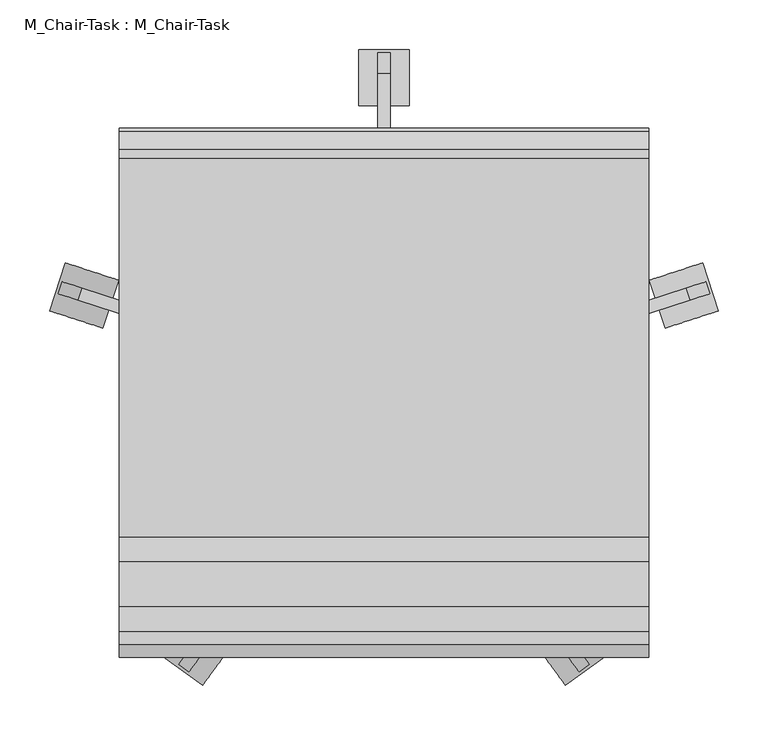
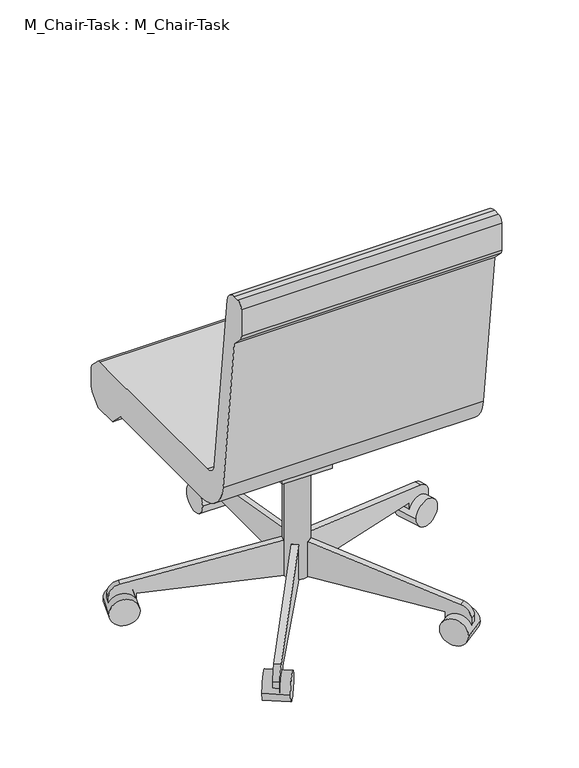
"""IFC4 building model written with IfcOpenShell, lengths in millimetres: furniture geometry, M_Chair-Task : M_Chair-Task."""

from ifc_helpers import new_model, si_unit, point, frame, frame_2d, origin, place, context, project, spatial, polyline, circle_curve, trimmed, segment, composite_curve, outline, extrude, source, transform, mapped, element, save


def m_chair_task_m_chair_task_9903d5c1(model_context):
    return source(origin(), model_context, "Body", "SweptSolid", [
        extrude(outline(composite_curve([segment(polyline([(-126.2050455, 457.2), (255.0102301, 457.2)]), True, "CONTINUOUS"), segment(trimmed(circle_curve(frame_2d((255.0102301, 444.5)), 12.7), [point((255.0102301, 457.2))], [point((263.9604301, 453.510212))], False, "CARTESIAN"), True, "CONTINUOUS"), segment(polyline([(263.9604301, 453.510212), (281.8961016, 435.6939999)]), True, "CONTINUOUS"), segment(trimmed(circle_curve(frame_2d((272.9459016, 426.6837879)), 12.7), [point((281.8961016, 435.6939999))], [point((285.6459016, 426.6837879))], False, "CARTESIAN"), True, "CONTINUOUS"), segment(polyline([(285.6459016, 426.6837879), (285.6459016, 391.6405184)]), True, "CONTINUOUS"), segment(trimmed(circle_curve(frame_2d((260.2459016, 391.6405184)), 25.4), [point((285.6459016, 391.6405184))], [point((278.2663256, 373.7401184))], False, "CARTESIAN"), True, "CONTINUOUS"), segment(polyline([(278.2663256, 373.7401184), (260.2470284, 355.6), (209.4470284, 355.6), (181.0744602, 383.7835944), (-107.1089978, 383.7835944)]), True, "CONTINUOUS"), segment(trimmed(circle_curve(frame_2d((-107.1089978, 459.9835944)), 76.2), [point((-107.1089978, 383.7835944))], [point((-182.7870738, 451.0802913))], False, "CARTESIAN"), True, "CONTINUOUS"), segment(polyline([(-182.7870738, 451.0802913), (-222.3540984, 787.4), (-244.0343545, 809.0802561)]), True, "CONTINUOUS"), segment(trimmed(circle_curve(frame_2d((-235.0540984, 818.0605122)), 12.7), [point((-244.0343545, 809.0802561))], [point((-247.7540984, 818.0605122))], False, "CARTESIAN"), True, "CONTINUOUS"), segment(polyline([(-247.7540984, 818.0605122), (-247.7540984, 876.3)]), True, "CONTINUOUS"), segment(trimmed(circle_curve(frame_2d((-235.0540984, 876.3)), 12.7), [point((-247.7540984, 876.3))], [point((-235.0540984, 889.0))], False, "CARTESIAN"), True, "CONTINUOUS"), segment(polyline([(-235.0540984, 889.0), (-222.1789239, 889.0)]), True, "CONTINUOUS"), segment(trimmed(circle_curve(frame_2d((-222.1789239, 863.6)), 25.4), [point((-222.1789239, 889.0))], [point((-196.9528985, 866.5677677))], False, "CARTESIAN"), True, "CONTINUOUS"), segment(polyline([(-196.9528985, 866.5677677), (-151.4310708, 479.6322323)]), True, "CONTINUOUS"), segment(trimmed(circle_curve(frame_2d((-126.2050455, 482.6)), 25.4), [point((-151.4310708, 479.6322323))], [point((-126.2050455, 457.2))], True, "CARTESIAN"), True, "CONTINUOUS")], self_intersect=False)), frame((-125.7091803, 0.0, 0.0), z_axis=(1.0, 0.0, 0.0), x_axis=(0.0, 1.0, 0.0)), (0.0, 0.0, 1.0), 533.4),
        extrude(outline(polyline([(69.7459016, 383.7835944), (69.7459016, 371.0835944), (18.9459016, 283.0954134), (-19.1540984, 283.0954134), (-19.1540984, 383.7835944), (69.7459016, 383.7835944)])), frame((90.1908197, 0.0, 0.0), z_axis=(1.0, 0.0, 0.0), x_axis=(0.0, 1.0, 0.0)), (0.0, 0.0, 1.0), 101.6),
        extrude(outline(composite_curve([segment(polyline([(311.0459016, 53.5835944), (18.9459016, 53.5835944), (18.9459016, 129.7835944), (44.3459016, 129.7835944), (340.8565654, 77.5007643)]), True, "CONTINUOUS"), segment(trimmed(circle_curve(frame_2d((336.4459016, 52.4866474)), 25.4), [point((340.8565654, 77.5007643))], [point((361.8459016, 52.4866474))], False, "CARTESIAN"), True, "CONTINUOUS"), segment(polyline([(361.8459016, 52.4866474), (361.8459016, 28.1835944), (311.0459016, 28.1835944), (311.0459016, 53.5835944)]), True, "CONTINUOUS")], self_intersect=False)), frame((134.6408197, 0.0, 0.0), z_axis=(1.0, 0.0, 0.0), x_axis=(0.0, 1.0, 0.0)), (0.0, 0.0, 1.0), 12.7),
        extrude(outline(composite_curve([segment(trimmed(circle_curve(frame_2d((336.4459016, 28.1835944)), 28.2002727), [point((308.2456289, 28.1835944))], [point((364.6461744, 28.1835944))], False, "CARTESIAN"), True, "CONTINUOUS"), segment(trimmed(circle_curve(frame_2d((336.4459016, 28.1835944)), 28.2002727), [point((364.6461744, 28.1835944))], [point((308.2456289, 28.1835944))], False, "CARTESIAN"), True, "CONTINUOUS")], self_intersect=False)), frame((115.5908197, 0.0, 0.0), z_axis=(1.0, 0.0, 0.0), x_axis=(0.0, 1.0, 0.0)), (0.0, 0.0, 1.0), 50.8),
        extrude(outline(composite_curve([segment(polyline([(25.4, 0.0), (25.4, 292.1000001), (101.6, 292.1000001), (101.6, 266.7), (49.3171699, -29.8106636)]), True, "CONTINUOUS"), segment(trimmed(circle_curve(frame_2d((24.303053, -25.4)), 25.4), [point((49.3171699, -29.8106636))], [point((24.303053, -50.8))], False, "CARTESIAN"), True, "CONTINUOUS"), segment(polyline([(24.303053, -50.8), (0.0, -50.8), (0.0, 0.0), (25.4, 0.0)]), True, "CONTINUOUS")], self_intersect=False)), frame((-138.7750467, 103.1705568, 28.1835944), z_axis=(0.3090169943749487, 0.9510565162951532, 0.0), x_axis=(0.0, 0.0, 1.0)), (0.0, 0.0, 1.0), 12.7),
        extrude(outline(composite_curve([segment(trimmed(circle_curve(frame_2d((0.0, -28.2002727)), 28.2002727), [point((0.0, -56.4005454))], [point((0.0, 0.0))], False, "CARTESIAN"), True, "CONTINUOUS"), segment(trimmed(circle_curve(frame_2d((0.0, -28.2002727)), 28.2002727), [point((0.0, 0.0))], [point((0.0, -56.4005454))], False, "CARTESIAN"), True, "CONTINUOUS")], self_intersect=False)), frame((-195.638709, 101.6163254, 28.1835944), z_axis=(0.3090169943749487, 0.9510565162951532, 0.0), x_axis=(0.0, 0.0, -1.0)), (0.0, 0.0, 1.0), 50.8),
        extrude(outline(composite_curve([segment(polyline([(25.4, 0.0), (25.4, 292.1), (101.6, 292.1), (101.6, 266.7), (49.3171699, -29.8106637)]), True, "CONTINUOUS"), segment(trimmed(circle_curve(frame_2d((24.303053, -25.3999999)), 25.4), [point((49.3171699, -29.8106637))], [point((24.303053, -50.8))], False, "CARTESIAN"), True, "CONTINUOUS"), segment(polyline([(24.303053, -50.8), (0.0, -50.8), (0.0, 0.0), (25.4, 0.0)]), True, "CONTINUOUS")], self_intersect=False)), frame((-25.5639946, -221.1003988, 28.1835944), z_axis=(-0.8090169943749459, 0.5877852522924754, 0.0), x_axis=(0.0, 0.0, 1.0)), (0.0, 0.0, 1.0), 12.7),
        extrude(outline(composite_curve([segment(trimmed(circle_curve(frame_2d((0.0, -28.2002727)), 28.2002727), [point((0.0, -56.4005455))], [point((0.0, 0.0))], False, "CARTESIAN"), True, "CONTINUOUS"), segment(trimmed(circle_curve(frame_2d((0.0, -28.2002727)), 28.2002727), [point((0.0, 0.0))], [point((0.0, -56.4005455))], False, "CARTESIAN"), True, "CONTINUOUS")], self_intersect=False)), frame((-41.6576707, -275.6612394, 28.1835944), z_axis=(-0.8090169943749458, 0.5877852522924754, 0.0), x_axis=(0.0, 0.0, -1.0)), (0.0, 0.0, 1.0), 50.8),
        extrude(outline(composite_curve([segment(polyline([(-25.4, 0.0), (0.0, 0.0), (0.0, -50.8), (-24.303053, -50.8)]), True, "CONTINUOUS"), segment(trimmed(circle_curve(frame_2d((-24.303053, -25.3999999)), 25.4), [point((-24.303053, -50.8))], [point((-49.3171699, -29.8106636))], False, "CARTESIAN"), True, "CONTINUOUS"), segment(polyline([(-49.3171699, -29.8106636), (-101.6, 266.7), (-101.6, 292.1), (-25.4, 292.1), (-25.4, 0.0)]), True, "CONTINUOUS")], self_intersect=False)), frame((307.545634, -221.1003988, 28.1835944), z_axis=(0.8090169943749499, 0.5877852522924699, 0.0), x_axis=(0.0, 0.0, -1.0)), (0.0, 0.0, 1.0), 12.7),
        extrude(outline(composite_curve([segment(trimmed(circle_curve(frame_2d((0.0, -28.2002727)), 28.2002727), [point((0.0, -56.4005455))], [point((0.0, 0.0))], False, "CARTESIAN"), True, "CONTINUOUS"), segment(trimmed(circle_curve(frame_2d((0.0, -28.2002727)), 28.2002727), [point((0.0, 0.0))], [point((0.0, -56.4005455))], False, "CARTESIAN"), True, "CONTINUOUS")], self_intersect=False)), frame((323.63931, -275.6612394, 28.1835944), z_axis=(0.8090169943749499, 0.5877852522924699, 0.0), x_axis=(0.0, 0.0, 1.0)), (0.0, 0.0, 1.0), 50.8),
        extrude(outline(composite_curve([segment(polyline([(-25.4, 0.0), (0.0, 0.0), (0.0, -50.8), (-24.303053, -50.8)]), True, "CONTINUOUS"), segment(trimmed(circle_curve(frame_2d((-24.303053, -25.4)), 25.4), [point((-24.303053, -50.8))], [point((-49.3171699, -29.8106637))], False, "CARTESIAN"), True, "CONTINUOUS"), segment(polyline([(-49.3171699, -29.8106637), (-101.6, 266.7), (-101.6, 292.1), (-25.4, 292.1), (-25.4, 0.0)]), True, "CONTINUOUS")], self_intersect=False)), frame((420.756686, 103.1705568, 28.1835944), z_axis=(-0.3090169943749423, 0.9510565162951553, 0.0), x_axis=(0.0, 0.0, -1.0)), (0.0, 0.0, 1.0), 12.7),
        extrude(outline(composite_curve([segment(trimmed(circle_curve(frame_2d((0.0, -28.2002727)), 28.2002727), [point((0.0, -56.4005455))], [point((0.0, 0.0))], False, "CARTESIAN"), True, "CONTINUOUS"), segment(trimmed(circle_curve(frame_2d((0.0, -28.2002727)), 28.2002727), [point((0.0, 0.0))], [point((0.0, -56.4005455))], False, "CARTESIAN"), True, "CONTINUOUS")], self_intersect=False)), frame((477.6203484, 101.6163254, 28.1835944), z_axis=(-0.3090169943749423, 0.9510565162951553, 0.0), x_axis=(0.0, 0.0, 1.0)), (0.0, 0.0, 1.0), 50.8),
        extrude(outline(composite_curve([segment(trimmed(circle_curve(frame_2d((140.9908197, 18.9459016)), 25.4), [point((115.5908197, 18.9459016))], [point((166.3908197, 18.9459016))], False, "CARTESIAN"), True, "CONTINUOUS"), segment(trimmed(circle_curve(frame_2d((140.9908197, 18.9459016)), 25.4), [point((166.3908197, 18.9459016))], [point((115.5908197, 18.9459016))], False, "CARTESIAN"), True, "CONTINUOUS")], self_intersect=False)), frame((0.0, 0.0, 53.5835944), z_axis=(0.0, 0.0, 1.0), x_axis=(1.0, 0.0, 0.0)), (0.0, 0.0, 1.0), 330.5914056),
    ])


if __name__ == "__main__":
    model = new_model("IFC4")
    model_context = context("Model", 3, world=origin())
    ifc_project = project(units=[si_unit("LENGTHUNIT", "METRE", prefix="MILLI")], contexts=[model_context])
    site = spatial("IfcSite", under=ifc_project)
    building = spatial("IfcBuilding", under=site)
    placement = place(None, origin())
    m_chair_task_m_chair_task_shape = m_chair_task_m_chair_task_9903d5c1(model_context)
    element("IfcFurniture", 1, ObjectType="M_Chair-Task : M_Chair-Task", at=placement, inside=building, context=model_context, shape_type="MappedRepresentation", body=[
        mapped(m_chair_task_m_chair_task_shape, transform((0.0, 0.0, 0.0), x_axis=(1.0, 0.0, 0.0), y_axis=(0.0, 1.0, 0.0), z_axis=(0.0, 0.0, 1.0))),
    ])
    save(model, "model.ifc")

# Revit data of these elements
# Type "M_Chair-Task : M_Chair-Task"
#   Base Material = Plastic, Opaque Black
#   Caster Material = Plastic, Opaque Black
#   Seat/Back Material = Textile - Slate Blue
#   Default Elevation = 0
# Element 1 (IfcFurniture, "M_Chair-Task : M_Chair-Task")
#   Materials on its faces: "Plastic, Opaque Black", "Textile - Slate Blue"
# Materials
#   "Plastic, Opaque Black": class "Plastic", colour RGB 0 0 0, transparency 0.7, Description = "Plastic, generic, opaque black", Cost = 0
#   "Textile - Slate Blue": class "Fabric", colour RGB 98 102 118, transparency 0
